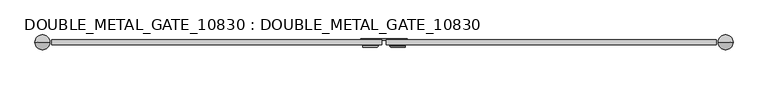
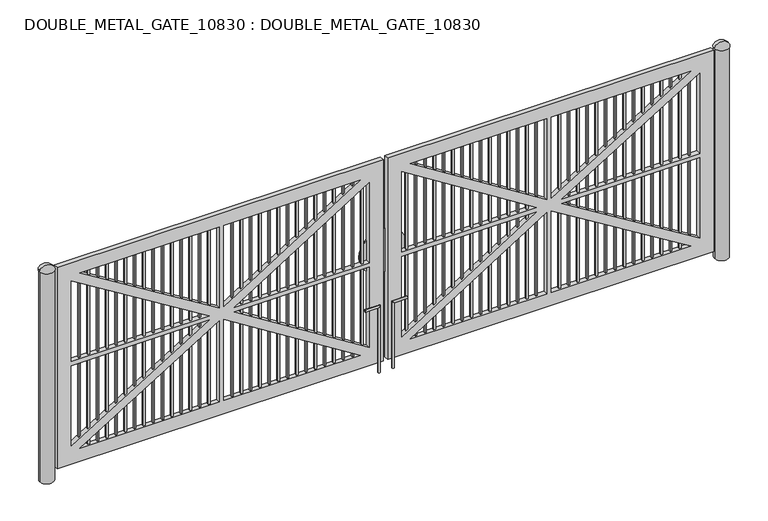
"""IFC4 building model written with IfcOpenShell, lengths in millimetres: proxy geometry, DOUBLE_METAL_GATE_10830 : DOUBLE_METAL_GATE_10830."""

from ifc_helpers import new_model, si_unit, point, frame, frame_2d, origin, origin_with_axes, place, context, project, spatial, polyline, circle_curve, ellipse_curve, trimmed, segment, composite_curve, outline, extrude, source, transform, mapped, element, save
from ifc_brep_helpers import plane_surface, cylinder_surface, revolved_surface, advanced_brep


def double_metal_gate_10830_double_metal_gate_10830_8bfe90f4(model_context):
    return source(origin(), model_context, "Body", "SolidModel", [
        extrude(outline(composite_curve([segment(trimmed(circle_curve(frame_2d((-4461.3106624, 76.2)), 76.2), [point((-4537.5106624, 76.2))], [point((-4385.1106624, 76.2))], False, "CARTESIAN"), True, "CONTINUOUS"), segment(trimmed(circle_curve(frame_2d((-4461.3106624, 76.2)), 76.2), [point((-4385.1106624, 76.2))], [point((-4537.5106624, 76.2))], False, "CARTESIAN"), True, "CONTINUOUS")], self_intersect=False)), origin_with_axes(), (0.0, 0.0, 1.0), 2438.4),
        advanced_brep(
        [(-4461.3106624, 76.2, 2489.2), (-4380.397889, 76.2, 2438.4), (-4542.2234359, 76.2, 2438.4), (-4461.3106624, 76.2, 2438.4)],
        [
            (0, 1, circle_curve(frame((-4456.7603117, 76.2, 2406.6099024), z_axis=(0.0, 1.0, 0.0), x_axis=(-1.0, 0.0, 0.0)), 82.7153547)),
            (1, 2, circle_curve(frame((-4461.3106624, 76.2, 2438.4), z_axis=(0.0, 0.0, 1.0), x_axis=(1.0, 0.0, 0.0)), 80.9127734)),
            (2, 0, circle_curve(frame((-4465.8610132, 76.2, 2406.6099024), z_axis=(0.0, 1.0, 0.0), x_axis=(1.0, 0.0, 0.0)), 82.7153547)),
            (2, 1, circle_curve(frame((-4461.3106624, 76.2, 2438.4), z_axis=(0.0, 0.0, 1.0), x_axis=(1.0, 0.0, 0.0)), 80.9127734)),
            (1, 3),
            (3, 2),
        ],
        [
            revolved_surface(trimmed(ellipse_curve(frame((-4456.7603117, 76.2, 2406.6099024), z_axis=(0.0, -1.0, 0.0), x_axis=(-1.0, 0.0, 0.0)), 82.7153547, 82.7153547), [point((-4380.397889, 76.2, 2438.4))], [point((-4461.3106624, 76.2, 2489.2))], True, "CARTESIAN"), (-4461.3106624, 76.2, 2438.4), (0.0, 0.0, 1.0)),
            plane_surface(frame((-4461.3106624, 76.2, 2438.4), z_axis=(0.0, 0.0, -1.0), x_axis=(1.0, 0.0, 0.0))),
        ],
        [
            (0, [[1, 2, 3]]),
            (0, [[-3, 4, -1]]),
            (1, [[-2, 5, 6]]),
            (1, [[-4, -6, -5]]),
        ],
    ),
        advanced_brep(
        [(2937.3106624, 76.2, 2489.2), (3018.2234359, 76.2, 2438.4), (2856.397889, 76.2, 2438.4), (2937.3106624, 76.2, 2438.4)],
        [
            (0, 1, circle_curve(frame((2941.8610132, 76.2, 2406.6099024), z_axis=(0.0, 1.0, 0.0), x_axis=(-1.0, 0.0, 0.0)), 82.7153547)),
            (1, 2, circle_curve(frame((2937.3106624, 76.2, 2438.4), z_axis=(0.0, 0.0, 1.0), x_axis=(1.0, 0.0, 0.0)), 80.9127734)),
            (2, 0, circle_curve(frame((2932.7603117, 76.2, 2406.6099024), z_axis=(0.0, 1.0, 0.0), x_axis=(1.0, 0.0, 0.0)), 82.7153547)),
            (2, 1, circle_curve(frame((2937.3106624, 76.2, 2438.4), z_axis=(0.0, 0.0, 1.0), x_axis=(1.0, 0.0, 0.0)), 80.9127734)),
            (1, 3),
            (3, 2),
        ],
        [
            revolved_surface(trimmed(ellipse_curve(frame((2941.8610132, 76.2, 2406.6099024), z_axis=(0.0, -1.0, 0.0), x_axis=(-1.0, 0.0, 0.0)), 82.7153547, 82.7153547), [point((3018.2234359, 76.2, 2438.4))], [point((2937.3106624, 76.2, 2489.2))], True, "CARTESIAN"), (2937.3106624, 76.2, 2438.4), (0.0, 0.0, 1.0)),
            plane_surface(frame((2937.3106624, 76.2, 2438.4), z_axis=(0.0, 0.0, -1.0), x_axis=(1.0, 0.0, 0.0))),
        ],
        [
            (0, [[1, 2, 3]]),
            (0, [[-3, 4, -1]]),
            (1, [[-2, 5, 6]]),
            (1, [[-4, -6, -5]]),
        ],
    ),
        extrude(outline(composite_curve([segment(trimmed(circle_curve(frame_2d((2937.3106624, 76.2)), 76.2), [point((3013.5106624, 76.2))], [point((2861.1106624, 76.2))], False, "CARTESIAN"), True, "CONTINUOUS"), segment(trimmed(circle_curve(frame_2d((2937.3106624, 76.2)), 76.2), [point((2861.1106624, 76.2))], [point((3013.5106624, 76.2))], False, "CARTESIAN"), True, "CONTINUOUS")], self_intersect=False)), origin_with_axes(), (0.0, 0.0, 1.0), 2438.4),
        extrude(outline(polyline([(101.6, -787.4), (2438.4, -787.4), (2438.4, -4359.7106624), (101.6, -4359.7106624), (101.6, -787.4)]), holes=[polyline([(2286.0, -1036.7285433), (1345.2791035, -2530.9106624), (2286.0, -2530.9106624), (2286.0, -1036.7285433)]), polyline([(2226.3516657, -4207.3106624), (1295.4, -2694.5142057), (1295.4, -4207.3106624), (2226.3516657, -4207.3106624)]), polyline([(2286.0, -2581.7106624), (1345.2791035, -2581.7106624), (2286.0, -4110.3821192), (2286.0, -2581.7106624)]), polyline([(1244.6, -4207.3106624), (1244.6, -2694.5142057), (313.6483343, -4207.3106624), (1244.6, -4207.3106624)]), polyline([(254.0, -2530.9106624), (1194.7208965, -2530.9106624), (254.0, -1036.7285433), (254.0, -2530.9106624)]), polyline([(1295.4, -939.8), (1295.4, -2418.1071192), (2226.3516657, -939.8), (1295.4, -939.8)]), polyline([(1244.6, -2418.1071192), (1244.6, -939.8), (313.6483343, -939.8), (1244.6, -2418.1071192)]), polyline([(1194.7208965, -2581.7106624), (254.0, -2581.7106624), (254.0, -4110.3821192), (1194.7208965, -2581.7106624)])]), frame((0.0, 50.8, 0.0), z_axis=(0.0, 1.0, 0.0), x_axis=(0.0, 0.0, 1.0)), (0.0, 0.0, 1.0), 50.8),
        extrude(outline(polyline([(-4096.1856624, 66.675), (-4115.2356624, 66.675), (-4115.2356624, 85.725), (-4096.1856624, 85.725), (-4096.1856624, 66.675)])), frame((0.0, 0.0, 254.0), z_axis=(0.0, 0.0, 1.0), x_axis=(1.0, 0.0, 0.0)), (0.0, 0.0, 1.0), 2032.0),
        extrude(outline(polyline([(-3994.5856624, 66.675), (-4013.6356624, 66.675), (-4013.6356624, 85.725), (-3994.5856624, 85.725), (-3994.5856624, 66.675)])), frame((0.0, 0.0, 254.0), z_axis=(0.0, 0.0, 1.0), x_axis=(1.0, 0.0, 0.0)), (0.0, 0.0, 1.0), 2032.0),
        extrude(outline(polyline([(-3892.9856624, 66.675), (-3912.0356624, 66.675), (-3912.0356624, 85.725), (-3892.9856624, 85.725), (-3892.9856624, 66.675)])), frame((0.0, 0.0, 254.0), z_axis=(0.0, 0.0, 1.0), x_axis=(1.0, 0.0, 0.0)), (0.0, 0.0, 1.0), 2032.0),
        extrude(outline(polyline([(-3791.3856624, 66.675), (-3810.4356624, 66.675), (-3810.4356624, 85.725), (-3791.3856624, 85.725), (-3791.3856624, 66.675)])), frame((0.0, 0.0, 254.0), z_axis=(0.0, 0.0, 1.0), x_axis=(1.0, 0.0, 0.0)), (0.0, 0.0, 1.0), 2032.0),
        extrude(outline(polyline([(-3689.7856624, 66.675), (-3708.8356624, 66.675), (-3708.8356624, 85.725), (-3689.7856624, 85.725), (-3689.7856624, 66.675)])), frame((0.0, 0.0, 254.0), z_axis=(0.0, 0.0, 1.0), x_axis=(1.0, 0.0, 0.0)), (0.0, 0.0, 1.0), 2032.0),
        extrude(outline(polyline([(-3588.1856624, 66.675), (-3607.2356624, 66.675), (-3607.2356624, 85.725), (-3588.1856624, 85.725), (-3588.1856624, 66.675)])), frame((0.0, 0.0, 254.0), z_axis=(0.0, 0.0, 1.0), x_axis=(1.0, 0.0, 0.0)), (0.0, 0.0, 1.0), 2032.0),
        extrude(outline(polyline([(-3486.5856624, 66.675), (-3505.6356624, 66.675), (-3505.6356624, 85.725), (-3486.5856624, 85.725), (-3486.5856624, 66.675)])), frame((0.0, 0.0, 254.0), z_axis=(0.0, 0.0, 1.0), x_axis=(1.0, 0.0, 0.0)), (0.0, 0.0, 1.0), 2032.0),
        extrude(outline(polyline([(-3384.9856624, 66.675), (-3404.0356624, 66.675), (-3404.0356624, 85.725), (-3384.9856624, 85.725), (-3384.9856624, 66.675)])), frame((0.0, 0.0, 254.0), z_axis=(0.0, 0.0, 1.0), x_axis=(1.0, 0.0, 0.0)), (0.0, 0.0, 1.0), 2032.0),
        extrude(outline(polyline([(-3283.3856624, 66.675), (-3302.4356624, 66.675), (-3302.4356624, 85.725), (-3283.3856624, 85.725), (-3283.3856624, 66.675)])), frame((0.0, 0.0, 254.0), z_axis=(0.0, 0.0, 1.0), x_axis=(1.0, 0.0, 0.0)), (0.0, 0.0, 1.0), 2032.0),
        extrude(outline(polyline([(-3181.7856624, 66.675), (-3200.8356624, 66.675), (-3200.8356624, 85.725), (-3181.7856624, 85.725), (-3181.7856624, 66.675)])), frame((0.0, 0.0, 254.0), z_axis=(0.0, 0.0, 1.0), x_axis=(1.0, 0.0, 0.0)), (0.0, 0.0, 1.0), 2032.0),
        extrude(outline(polyline([(-3080.1856624, 66.675), (-3099.2356624, 66.675), (-3099.2356624, 85.725), (-3080.1856624, 85.725), (-3080.1856624, 66.675)])), frame((0.0, 0.0, 254.0), z_axis=(0.0, 0.0, 1.0), x_axis=(1.0, 0.0, 0.0)), (0.0, 0.0, 1.0), 2032.0),
        extrude(outline(polyline([(-2978.5856624, 66.675), (-2997.6356624, 66.675), (-2997.6356624, 85.725), (-2978.5856624, 85.725), (-2978.5856624, 66.675)])), frame((0.0, 0.0, 254.0), z_axis=(0.0, 0.0, 1.0), x_axis=(1.0, 0.0, 0.0)), (0.0, 0.0, 1.0), 2032.0),
        extrude(outline(polyline([(-2876.9856624, 66.675), (-2896.0356624, 66.675), (-2896.0356624, 85.725), (-2876.9856624, 85.725), (-2876.9856624, 66.675)])), frame((0.0, 0.0, 254.0), z_axis=(0.0, 0.0, 1.0), x_axis=(1.0, 0.0, 0.0)), (0.0, 0.0, 1.0), 2032.0),
        extrude(outline(polyline([(-2775.3856624, 66.675), (-2794.4356624, 66.675), (-2794.4356624, 85.725), (-2775.3856624, 85.725), (-2775.3856624, 66.675)])), frame((0.0, 0.0, 254.0), z_axis=(0.0, 0.0, 1.0), x_axis=(1.0, 0.0, 0.0)), (0.0, 0.0, 1.0), 2032.0),
        extrude(outline(polyline([(-2673.7856624, 66.675), (-2692.8356624, 66.675), (-2692.8356624, 85.725), (-2673.7856624, 85.725), (-2673.7856624, 66.675)])), frame((0.0, 0.0, 254.0), z_axis=(0.0, 0.0, 1.0), x_axis=(1.0, 0.0, 0.0)), (0.0, 0.0, 1.0), 2032.0),
        extrude(outline(polyline([(-2419.7856624, 66.675), (-2438.8356624, 66.675), (-2438.8356624, 85.725), (-2419.7856624, 85.725), (-2419.7856624, 66.675)])), frame((0.0, 0.0, 254.0), z_axis=(0.0, 0.0, 1.0), x_axis=(1.0, 0.0, 0.0)), (0.0, 0.0, 1.0), 2032.0),
        extrude(outline(polyline([(-2318.1856624, 66.675), (-2337.2356624, 66.675), (-2337.2356624, 85.725), (-2318.1856624, 85.725), (-2318.1856624, 66.675)])), frame((0.0, 0.0, 254.0), z_axis=(0.0, 0.0, 1.0), x_axis=(1.0, 0.0, 0.0)), (0.0, 0.0, 1.0), 2032.0),
        extrude(outline(polyline([(-2216.5856624, 66.675), (-2235.6356624, 66.675), (-2235.6356624, 85.725), (-2216.5856624, 85.725), (-2216.5856624, 66.675)])), frame((0.0, 0.0, 254.0), z_axis=(0.0, 0.0, 1.0), x_axis=(1.0, 0.0, 0.0)), (0.0, 0.0, 1.0), 2032.0),
        extrude(outline(polyline([(-2114.9856624, 66.675), (-2134.0356624, 66.675), (-2134.0356624, 85.725), (-2114.9856624, 85.725), (-2114.9856624, 66.675)])), frame((0.0, 0.0, 254.0), z_axis=(0.0, 0.0, 1.0), x_axis=(1.0, 0.0, 0.0)), (0.0, 0.0, 1.0), 2032.0),
        extrude(outline(polyline([(-2013.3856624, 66.675), (-2032.4356624, 66.675), (-2032.4356624, 85.725), (-2013.3856624, 85.725), (-2013.3856624, 66.675)])), frame((0.0, 0.0, 254.0), z_axis=(0.0, 0.0, 1.0), x_axis=(1.0, 0.0, 0.0)), (0.0, 0.0, 1.0), 2032.0),
        extrude(outline(polyline([(-1911.7856624, 66.675), (-1930.8356624, 66.675), (-1930.8356624, 85.725), (-1911.7856624, 85.725), (-1911.7856624, 66.675)])), frame((0.0, 0.0, 254.0), z_axis=(0.0, 0.0, 1.0), x_axis=(1.0, 0.0, 0.0)), (0.0, 0.0, 1.0), 2032.0),
        extrude(outline(polyline([(-1810.1856624, 66.675), (-1829.2356624, 66.675), (-1829.2356624, 85.725), (-1810.1856624, 85.725), (-1810.1856624, 66.675)])), frame((0.0, 0.0, 254.0), z_axis=(0.0, 0.0, 1.0), x_axis=(1.0, 0.0, 0.0)), (0.0, 0.0, 1.0), 2032.0),
        extrude(outline(polyline([(-1708.5856624, 66.675), (-1727.6356624, 66.675), (-1727.6356624, 85.725), (-1708.5856624, 85.725), (-1708.5856624, 66.675)])), frame((0.0, 0.0, 254.0), z_axis=(0.0, 0.0, 1.0), x_axis=(1.0, 0.0, 0.0)), (0.0, 0.0, 1.0), 2032.0),
        extrude(outline(polyline([(-1606.9856624, 66.675), (-1626.0356624, 66.675), (-1626.0356624, 85.725), (-1606.9856624, 85.725), (-1606.9856624, 66.675)])), frame((0.0, 0.0, 254.0), z_axis=(0.0, 0.0, 1.0), x_axis=(1.0, 0.0, 0.0)), (0.0, 0.0, 1.0), 2032.0),
        extrude(outline(polyline([(-1505.3856624, 66.675), (-1524.4356624, 66.675), (-1524.4356624, 85.725), (-1505.3856624, 85.725), (-1505.3856624, 66.675)])), frame((0.0, 0.0, 254.0), z_axis=(0.0, 0.0, 1.0), x_axis=(1.0, 0.0, 0.0)), (0.0, 0.0, 1.0), 2032.0),
        extrude(outline(polyline([(-1403.7856624, 66.675), (-1422.8356624, 66.675), (-1422.8356624, 85.725), (-1403.7856624, 85.725), (-1403.7856624, 66.675)])), frame((0.0, 0.0, 254.0), z_axis=(0.0, 0.0, 1.0), x_axis=(1.0, 0.0, 0.0)), (0.0, 0.0, 1.0), 2032.0),
        extrude(outline(polyline([(-1302.1856624, 66.675), (-1321.2356624, 66.675), (-1321.2356624, 85.725), (-1302.1856624, 85.725), (-1302.1856624, 66.675)])), frame((0.0, 0.0, 254.0), z_axis=(0.0, 0.0, 1.0), x_axis=(1.0, 0.0, 0.0)), (0.0, 0.0, 1.0), 2032.0),
        extrude(outline(polyline([(-1200.5856624, 66.675), (-1219.6356624, 66.675), (-1219.6356624, 85.725), (-1200.5856624, 85.725), (-1200.5856624, 66.675)])), frame((0.0, 0.0, 254.0), z_axis=(0.0, 0.0, 1.0), x_axis=(1.0, 0.0, 0.0)), (0.0, 0.0, 1.0), 2032.0),
        extrude(outline(polyline([(-1098.9856624, 66.675), (-1118.0356624, 66.675), (-1118.0356624, 85.725), (-1098.9856624, 85.725), (-1098.9856624, 66.675)])), frame((0.0, 0.0, 254.0), z_axis=(0.0, 0.0, 1.0), x_axis=(1.0, 0.0, 0.0)), (0.0, 0.0, 1.0), 2032.0),
        extrude(outline(polyline([(-997.3856624, 66.675), (-1016.4356624, 66.675), (-1016.4356624, 85.725), (-997.3856624, 85.725), (-997.3856624, 66.675)])), frame((0.0, 0.0, 254.0), z_axis=(0.0, 0.0, 1.0), x_axis=(1.0, 0.0, 0.0)), (0.0, 0.0, 1.0), 2032.0),
        extrude(outline(polyline([(101.6, -736.6), (101.6, 2835.7106624), (2438.4, 2835.7106624), (2438.4, -736.6), (101.6, -736.6)]), holes=[polyline([(2286.0, 1057.7106624), (2286.0, 2586.3821192), (1345.2791035, 1057.7106624), (2286.0, 1057.7106624)]), polyline([(1295.4, -584.2), (2226.3516657, -584.2), (1295.4, 894.1071192), (1295.4, -584.2)]), polyline([(254.0, 1006.9106624), (254.0, -487.2714567), (1194.7208965, 1006.9106624), (254.0, 1006.9106624)]), polyline([(1244.6, 2683.3106624), (313.6483343, 2683.3106624), (1244.6, 1170.5142057), (1244.6, 2683.3106624)]), polyline([(1194.7208965, 1057.7106624), (254.0, 2586.3821192), (254.0, 1057.7106624), (1194.7208965, 1057.7106624)]), polyline([(1244.6, 894.1071192), (313.6483343, -584.2), (1244.6, -584.2), (1244.6, 894.1071192)]), polyline([(2286.0, -487.2714567), (2286.0, 1006.9106624), (1345.2791035, 1006.9106624), (2286.0, -487.2714567)]), polyline([(2226.3516657, 2683.3106624), (1295.4, 2683.3106624), (1295.4, 1170.5142057), (2226.3516657, 2683.3106624)])]), frame((0.0, 50.8, 0.0), z_axis=(0.0, 1.0, 0.0), x_axis=(0.0, 0.0, 1.0)), (0.0, 0.0, 1.0), 50.8),
        extrude(outline(composite_curve([segment(trimmed(circle_curve(frame_2d((1342.973777, -762.0)), 254.0), [point((1342.973777, -1016.0))], [point((1342.973777, -508.0))], False, "CARTESIAN"), True, "CONTINUOUS"), segment(trimmed(circle_curve(frame_2d((1342.973777, -762.0)), 254.0), [point((1342.973777, -508.0))], [point((1342.973777, -1016.0))], False, "CARTESIAN"), True, "CONTINUOUS")], self_intersect=False)), frame((0.0, 101.6, 0.0), z_axis=(0.0, 1.0, 0.0), x_axis=(0.0, 0.0, 1.0)), (0.0, 0.0, 1.0), 12.7),
        extrude(outline(polyline([(2572.1856624, 66.675), (2572.1856624, 85.725), (2591.2356624, 85.725), (2591.2356624, 66.675), (2572.1856624, 66.675)])), frame((0.0, 0.0, 254.0), z_axis=(0.0, 0.0, 1.0), x_axis=(1.0, 0.0, 0.0)), (0.0, 0.0, 1.0), 2032.0),
        extrude(outline(polyline([(2470.5856624, 66.675), (2470.5856624, 85.725), (2489.6356624, 85.725), (2489.6356624, 66.675), (2470.5856624, 66.675)])), frame((0.0, 0.0, 254.0), z_axis=(0.0, 0.0, 1.0), x_axis=(1.0, 0.0, 0.0)), (0.0, 0.0, 1.0), 2032.0),
        extrude(outline(polyline([(2368.9856624, 66.675), (2368.9856624, 85.725), (2388.0356624, 85.725), (2388.0356624, 66.675), (2368.9856624, 66.675)])), frame((0.0, 0.0, 254.0), z_axis=(0.0, 0.0, 1.0), x_axis=(1.0, 0.0, 0.0)), (0.0, 0.0, 1.0), 2032.0),
        extrude(outline(polyline([(2267.3856624, 66.675), (2267.3856624, 85.725), (2286.4356624, 85.725), (2286.4356624, 66.675), (2267.3856624, 66.675)])), frame((0.0, 0.0, 254.0), z_axis=(0.0, 0.0, 1.0), x_axis=(1.0, 0.0, 0.0)), (0.0, 0.0, 1.0), 2032.0),
        extrude(outline(polyline([(2165.7856624, 66.675), (2165.7856624, 85.725), (2184.8356624, 85.725), (2184.8356624, 66.675), (2165.7856624, 66.675)])), frame((0.0, 0.0, 254.0), z_axis=(0.0, 0.0, 1.0), x_axis=(1.0, 0.0, 0.0)), (0.0, 0.0, 1.0), 2032.0),
        extrude(outline(polyline([(2064.1856624, 66.675), (2064.1856624, 85.725), (2083.2356624, 85.725), (2083.2356624, 66.675), (2064.1856624, 66.675)])), frame((0.0, 0.0, 254.0), z_axis=(0.0, 0.0, 1.0), x_axis=(1.0, 0.0, 0.0)), (0.0, 0.0, 1.0), 2032.0),
        extrude(outline(polyline([(1962.5856624, 66.675), (1962.5856624, 85.725), (1981.6356624, 85.725), (1981.6356624, 66.675), (1962.5856624, 66.675)])), frame((0.0, 0.0, 254.0), z_axis=(0.0, 0.0, 1.0), x_axis=(1.0, 0.0, 0.0)), (0.0, 0.0, 1.0), 2032.0),
        extrude(outline(polyline([(1860.9856624, 66.675), (1860.9856624, 85.725), (1880.0356624, 85.725), (1880.0356624, 66.675), (1860.9856624, 66.675)])), frame((0.0, 0.0, 254.0), z_axis=(0.0, 0.0, 1.0), x_axis=(1.0, 0.0, 0.0)), (0.0, 0.0, 1.0), 2032.0),
        extrude(outline(polyline([(1759.3856624, 66.675), (1759.3856624, 85.725), (1778.4356624, 85.725), (1778.4356624, 66.675), (1759.3856624, 66.675)])), frame((0.0, 0.0, 254.0), z_axis=(0.0, 0.0, 1.0), x_axis=(1.0, 0.0, 0.0)), (0.0, 0.0, 1.0), 2032.0),
        extrude(outline(polyline([(1657.7856624, 66.675), (1657.7856624, 85.725), (1676.8356624, 85.725), (1676.8356624, 66.675), (1657.7856624, 66.675)])), frame((0.0, 0.0, 254.0), z_axis=(0.0, 0.0, 1.0), x_axis=(1.0, 0.0, 0.0)), (0.0, 0.0, 1.0), 2032.0),
        extrude(outline(polyline([(1556.1856624, 66.675), (1556.1856624, 85.725), (1575.2356624, 85.725), (1575.2356624, 66.675), (1556.1856624, 66.675)])), frame((0.0, 0.0, 254.0), z_axis=(0.0, 0.0, 1.0), x_axis=(1.0, 0.0, 0.0)), (0.0, 0.0, 1.0), 2032.0),
        extrude(outline(polyline([(1454.5856624, 66.675), (1454.5856624, 85.725), (1473.6356624, 85.725), (1473.6356624, 66.675), (1454.5856624, 66.675)])), frame((0.0, 0.0, 254.0), z_axis=(0.0, 0.0, 1.0), x_axis=(1.0, 0.0, 0.0)), (0.0, 0.0, 1.0), 2032.0),
        extrude(outline(polyline([(1352.9856624, 66.675), (1352.9856624, 85.725), (1372.0356624, 85.725), (1372.0356624, 66.675), (1352.9856624, 66.675)])), frame((0.0, 0.0, 254.0), z_axis=(0.0, 0.0, 1.0), x_axis=(1.0, 0.0, 0.0)), (0.0, 0.0, 1.0), 2032.0),
        extrude(outline(polyline([(1251.3856624, 66.675), (1251.3856624, 85.725), (1270.4356624, 85.725), (1270.4356624, 66.675), (1251.3856624, 66.675)])), frame((0.0, 0.0, 254.0), z_axis=(0.0, 0.0, 1.0), x_axis=(1.0, 0.0, 0.0)), (0.0, 0.0, 1.0), 2032.0),
        extrude(outline(polyline([(1149.7856624, 66.675), (1149.7856624, 85.725), (1168.8356624, 85.725), (1168.8356624, 66.675), (1149.7856624, 66.675)])), frame((0.0, 0.0, 254.0), z_axis=(0.0, 0.0, 1.0), x_axis=(1.0, 0.0, 0.0)), (0.0, 0.0, 1.0), 2032.0),
        extrude(outline(polyline([(895.7856624, 66.675), (895.7856624, 85.725), (914.8356624, 85.725), (914.8356624, 66.675), (895.7856624, 66.675)])), frame((0.0, 0.0, 254.0), z_axis=(0.0, 0.0, 1.0), x_axis=(1.0, 0.0, 0.0)), (0.0, 0.0, 1.0), 2032.0),
        extrude(outline(polyline([(794.1856624, 66.675), (794.1856624, 85.725), (813.2356624, 85.725), (813.2356624, 66.675), (794.1856624, 66.675)])), frame((0.0, 0.0, 254.0), z_axis=(0.0, 0.0, 1.0), x_axis=(1.0, 0.0, 0.0)), (0.0, 0.0, 1.0), 2032.0),
        extrude(outline(polyline([(692.5856624, 66.675), (692.5856624, 85.725), (711.6356624, 85.725), (711.6356624, 66.675), (692.5856624, 66.675)])), frame((0.0, 0.0, 254.0), z_axis=(0.0, 0.0, 1.0), x_axis=(1.0, 0.0, 0.0)), (0.0, 0.0, 1.0), 2032.0),
        extrude(outline(polyline([(590.9856624, 66.675), (590.9856624, 85.725), (610.0356624, 85.725), (610.0356624, 66.675), (590.9856624, 66.675)])), frame((0.0, 0.0, 254.0), z_axis=(0.0, 0.0, 1.0), x_axis=(1.0, 0.0, 0.0)), (0.0, 0.0, 1.0), 2032.0),
        extrude(outline(polyline([(489.3856624, 66.675), (489.3856624, 85.725), (508.4356624, 85.725), (508.4356624, 66.675), (489.3856624, 66.675)])), frame((0.0, 0.0, 254.0), z_axis=(0.0, 0.0, 1.0), x_axis=(1.0, 0.0, 0.0)), (0.0, 0.0, 1.0), 2032.0),
        extrude(outline(polyline([(387.7856624, 66.675), (387.7856624, 85.725), (406.8356624, 85.725), (406.8356624, 66.675), (387.7856624, 66.675)])), frame((0.0, 0.0, 254.0), z_axis=(0.0, 0.0, 1.0), x_axis=(1.0, 0.0, 0.0)), (0.0, 0.0, 1.0), 2032.0),
        extrude(outline(polyline([(286.1856624, 66.675), (286.1856624, 85.725), (305.2356624, 85.725), (305.2356624, 66.675), (286.1856624, 66.675)])), frame((0.0, 0.0, 254.0), z_axis=(0.0, 0.0, 1.0), x_axis=(1.0, 0.0, 0.0)), (0.0, 0.0, 1.0), 2032.0),
        extrude(outline(polyline([(184.5856624, 66.675), (184.5856624, 85.725), (203.6356624, 85.725), (203.6356624, 66.675), (184.5856624, 66.675)])), frame((0.0, 0.0, 254.0), z_axis=(0.0, 0.0, 1.0), x_axis=(1.0, 0.0, 0.0)), (0.0, 0.0, 1.0), 2032.0),
        extrude(outline(polyline([(82.9856624, 66.675), (82.9856624, 85.725), (102.0356624, 85.725), (102.0356624, 66.675), (82.9856624, 66.675)])), frame((0.0, 0.0, 254.0), z_axis=(0.0, 0.0, 1.0), x_axis=(1.0, 0.0, 0.0)), (0.0, 0.0, 1.0), 2032.0),
        extrude(outline(polyline([(-18.6143376, 66.675), (-18.6143376, 85.725), (0.4356624, 85.725), (0.4356624, 66.675), (-18.6143376, 66.675)])), frame((0.0, 0.0, 254.0), z_axis=(0.0, 0.0, 1.0), x_axis=(1.0, 0.0, 0.0)), (0.0, 0.0, 1.0), 2032.0),
        extrude(outline(polyline([(-120.2143376, 66.675), (-120.2143376, 85.725), (-101.1643376, 85.725), (-101.1643376, 66.675), (-120.2143376, 66.675)])), frame((0.0, 0.0, 254.0), z_axis=(0.0, 0.0, 1.0), x_axis=(1.0, 0.0, 0.0)), (0.0, 0.0, 1.0), 2032.0),
        extrude(outline(polyline([(-221.8143376, 66.675), (-221.8143376, 85.725), (-202.7643376, 85.725), (-202.7643376, 66.675), (-221.8143376, 66.675)])), frame((0.0, 0.0, 254.0), z_axis=(0.0, 0.0, 1.0), x_axis=(1.0, 0.0, 0.0)), (0.0, 0.0, 1.0), 2032.0),
        extrude(outline(polyline([(-323.4143376, 66.675), (-323.4143376, 85.725), (-304.3643376, 85.725), (-304.3643376, 66.675), (-323.4143376, 66.675)])), frame((0.0, 0.0, 254.0), z_axis=(0.0, 0.0, 1.0), x_axis=(1.0, 0.0, 0.0)), (0.0, 0.0, 1.0), 2032.0),
        extrude(outline(polyline([(-425.0143376, 66.675), (-425.0143376, 85.725), (-405.9643376, 85.725), (-405.9643376, 66.675), (-425.0143376, 66.675)])), frame((0.0, 0.0, 254.0), z_axis=(0.0, 0.0, 1.0), x_axis=(1.0, 0.0, 0.0)), (0.0, 0.0, 1.0), 2032.0),
        extrude(outline(polyline([(-526.6143376, 66.675), (-526.6143376, 85.725), (-507.5643376, 85.725), (-507.5643376, 66.675), (-526.6143376, 66.675)])), frame((0.0, 0.0, 254.0), z_axis=(0.0, 0.0, 1.0), x_axis=(1.0, 0.0, 0.0)), (0.0, 0.0, 1.0), 2032.0),
        advanced_brep(
        [(-825.5, 38.1, 0.0), (-850.9, 38.1, 0.0), (-825.5, 38.1, 774.7), (-850.9, 38.1, 749.3), (-990.6, 38.1, 774.7), (-990.6, 38.1, 749.3)],
        [
            (0, 1, circle_curve(frame((-838.2, 38.1, 0.0), z_axis=(0.0, 0.0, -1.0), x_axis=(-1.0, 0.0, 0.0)), 12.7)),
            (1, 0, circle_curve(frame((-838.2, 38.1, 0.0), z_axis=(0.0, 0.0, -1.0), x_axis=(-1.0, 0.0, 0.0)), 12.7)),
            (0, 2),
            (2, 3, ellipse_curve(frame((-838.2, 38.1, 762.0), z_axis=(0.7071067811865457, 0.0, -0.7071067811865493), x_axis=(-0.7071067811865493, 0.0, -0.7071067811865457)), 17.9605122, 12.7)),
            (3, 1),
            (3, 2, ellipse_curve(frame((-838.2, 38.1, 762.0), z_axis=(0.7071067811865457, 0.0, -0.7071067811865493), x_axis=(-0.7071067811865493, 0.0, -0.7071067811865457)), 17.9605122, 12.7)),
            (4, 5, circle_curve(frame((-990.6, 38.1, 762.0), z_axis=(-1.0, 0.0, 0.0), x_axis=(0.0, 0.0, -1.0)), 12.7)),
            (5, 4, circle_curve(frame((-990.6, 38.1, 762.0), z_axis=(-1.0, 0.0, 0.0), x_axis=(0.0, 0.0, -1.0)), 12.7)),
            (2, 4),
            (5, 3),
        ],
        [
            plane_surface(frame((-838.2, 50.8, 0.0), z_axis=(0.0, 0.0, -1.0), x_axis=(0.0, -1.0, 0.0))),
            cylinder_surface(frame((-838.2, 38.1, 0.0), z_axis=(0.0, 0.0, -1.0), x_axis=(-1.0, 0.0, 0.0)), 12.7),
            plane_surface(frame((-990.6, 50.8, 762.0), z_axis=(-1.0, 0.0, 0.0), x_axis=(0.0, -1.0, 0.0))),
            cylinder_surface(frame((-838.2, 38.1, 762.0), z_axis=(1.0, 0.0, 0.0), x_axis=(0.0, 0.0, -1.0)), 12.7),
        ],
        [
            (0, [[1, 2]]),
            (1, [[-1, 3, 4, 5]]),
            (1, [[-2, -5, 6, -3]]),
            (2, [[7, 8]]),
            (3, [[-4, 9, -8, 10]]),
            (3, [[-6, -10, -7, -9]]),
        ],
    ),
        advanced_brep(
        [(-673.1, 38.1, 0.0), (-698.5, 38.1, 0.0), (-698.5, 38.1, 774.7), (-673.1, 38.1, 749.3), (-533.4, 38.1, 749.3), (-533.4, 38.1, 774.7)],
        [
            (0, 1, circle_curve(frame((-685.8, 38.1, 0.0), z_axis=(0.0, 0.0, -1.0), x_axis=(-1.0, 0.0, 0.0)), 12.7)),
            (1, 0, circle_curve(frame((-685.8, 38.1, 0.0), z_axis=(0.0, 0.0, -1.0), x_axis=(-1.0, 0.0, 0.0)), 12.7)),
            (1, 2),
            (2, 3, ellipse_curve(frame((-685.8, 38.1, 762.0), z_axis=(-0.7071067811865601, 0.0, -0.7071067811865349), x_axis=(0.7071067811865349, 0.0, -0.7071067811865601)), 17.9605122, 12.7)),
            (3, 0),
            (3, 2, ellipse_curve(frame((-685.8, 38.1, 762.0), z_axis=(-0.7071067811865601, 0.0, -0.7071067811865349), x_axis=(0.7071067811865349, 0.0, -0.7071067811865601)), 17.9605122, 12.7)),
            (4, 5, circle_curve(frame((-533.4, 38.1, 762.0), z_axis=(1.0, 0.0, 0.0), x_axis=(0.0, 0.0, 1.0)), 12.7)),
            (5, 4, circle_curve(frame((-533.4, 38.1, 762.0), z_axis=(1.0, 0.0, 0.0), x_axis=(0.0, 0.0, 1.0)), 12.7)),
            (2, 5),
            (4, 3),
        ],
        [
            plane_surface(frame((-685.8, 50.8, 0.0), z_axis=(0.0, 0.0, -1.0), x_axis=(0.0, -1.0, 0.0))),
            cylinder_surface(frame((-685.8, 38.1, 0.0), z_axis=(0.0, 0.0, -1.0), x_axis=(-1.0, 0.0, 0.0)), 12.7),
            plane_surface(frame((-533.4, 50.8, 762.0), z_axis=(1.0, 0.0, 0.0), x_axis=(0.0, -1.0, 0.0))),
            cylinder_surface(frame((-685.8, 38.1, 762.0), z_axis=(-1.0, 0.0, 0.0), x_axis=(0.0, 0.0, 1.0)), 12.7),
        ],
        [
            (0, [[1, 2]]),
            (1, [[-2, 3, 4, 5]]),
            (1, [[-1, -5, 6, -3]]),
            (2, [[7, 8]]),
            (3, [[-4, 9, -7, 10]]),
            (3, [[-6, -10, -8, -9]]),
        ],
    ),
    ])


if __name__ == "__main__":
    model = new_model("IFC4")
    model_context = context("Model", 3, world=origin())
    ifc_project = project(units=[si_unit("LENGTHUNIT", "METRE", prefix="MILLI")], contexts=[model_context])
    site = spatial("IfcSite", under=ifc_project)
    building = spatial("IfcBuilding", under=site)
    placement = place(None, origin())
    double_metal_gate_10830_double_metal_gate_10830_shape = double_metal_gate_10830_double_metal_gate_10830_8bfe90f4(model_context)
    element("IfcBuildingElementProxy", 1, Name="DOUBLE_METAL_GATE_10830 : DOUBLE_METAL_GATE_10830", ObjectType="DOUBLE_METAL_GATE_10830 : DOUBLE_METAL_GATE_10830", at=placement, inside=building, context=model_context, shape_type="MappedRepresentation", body=[
        mapped(double_metal_gate_10830_double_metal_gate_10830_shape, transform((0.0, 0.0, 0.0), x_axis=(1.0, 0.0, 0.0), y_axis=(0.0, 1.0, 0.0), z_axis=(0.0, 0.0, 1.0))),
    ])
    save(model, "model.ifc")

# Revit data of these elements
# Type "DOUBLE_METAL_GATE_10830 : DOUBLE_METAL_GATE_10830"
#   WIDTH [instance default] = 24' - 0"
#   Default Elevation = 0
#   Assembly Code = ""
# Element 1 (IfcBuildingElementProxy, "DOUBLE_METAL_GATE_10830 : DOUBLE_METAL_GATE_10830")
#   WIDTH = 23' - 9.2843"
#   Materials on its faces: "Default"
# Materials
#   "Default": colour RGB 127 127 127, transparency 0, Cost = 0
